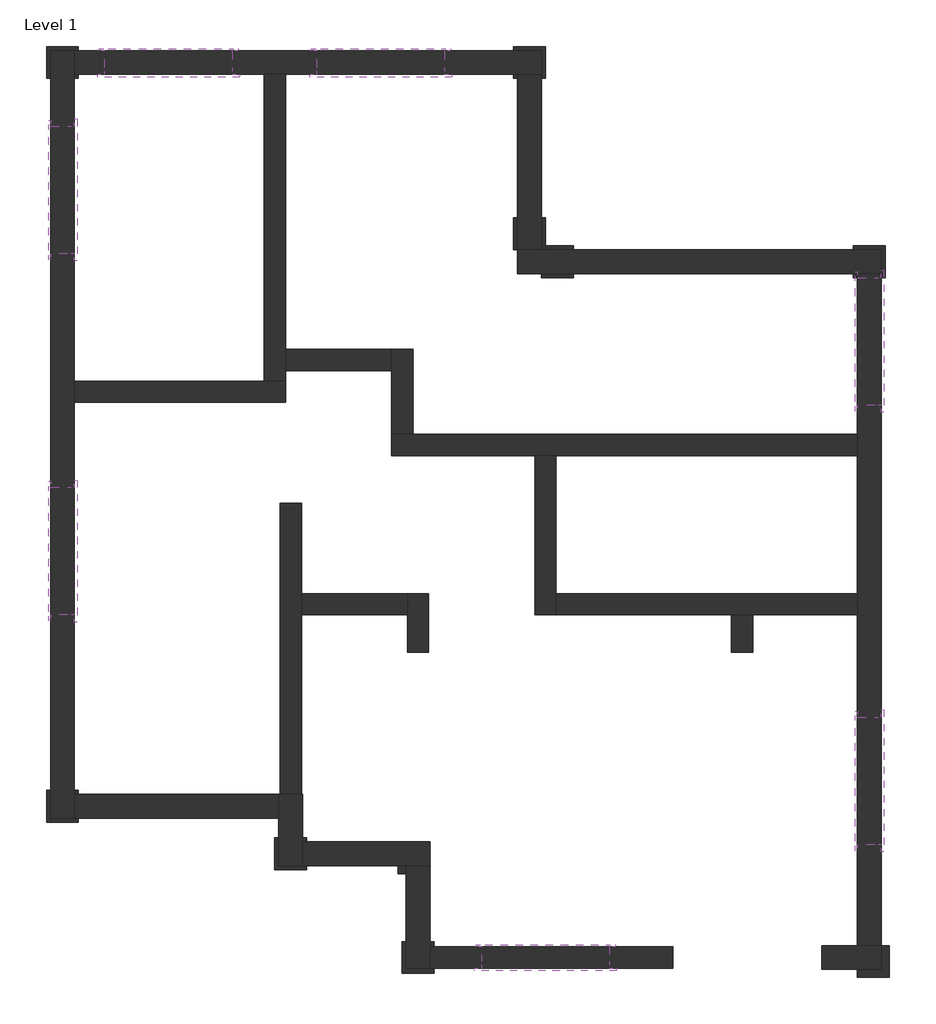
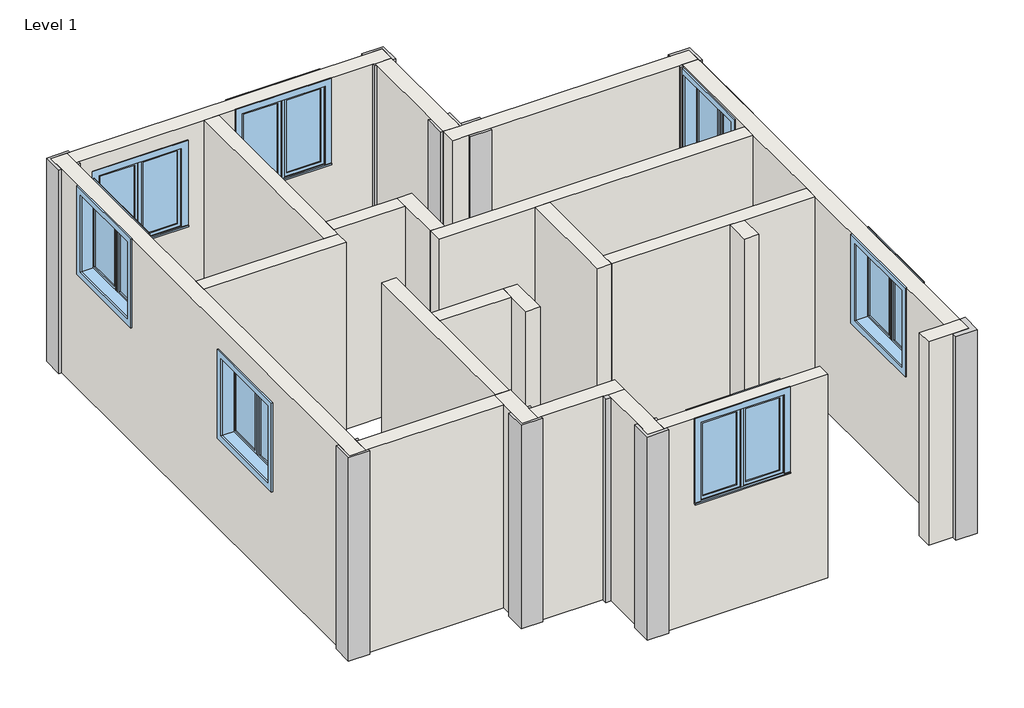
# One storey: 22 walls, 10 columns, 7 windows.
"""IFC4 building model written with IfcOpenShell, lengths in millimetres."""

from ifc_helpers import new_model, si_unit, origin, origin_with_axes, place, context, project, spatial, polyline, outline, extrude, faceted_brep, transform, mapped, element, save
from components import window_534dcd48, window_0862ab64

model = new_model("IFC4")

# Units and contexts
model_context = context("Model", 3, world=origin())
ifc_project = project(units=[si_unit("LENGTHUNIT", "METRE", prefix="MILLI")], contexts=[model_context])

# Site, building, storey
site = spatial("IfcSite", under=ifc_project)
building = spatial("IfcBuilding", under=site)
storey = spatial("IfcBuildingStorey", under=building, Name="Level 1", Elevation=0.0)

# Columns
placement = place(None, origin())
element("IfcColumn", 1, ObjectType="Rectangular Column : 12\" x 12\"", at=placement, inside=storey, context=model_context, shape_type="SweptSolid", body=[
    extrude(outline(polyline([(-12153.373418, 12563.7966667), (-12115.273418, 12563.7966667), (-12115.273418, 12525.6966667), (-12153.373418, 12525.6966667), (-12153.373418, 12563.7966667)])), origin_with_axes(), (0.0, 0.0, 1.0), 3048.0),
    extrude(outline(polyline([(-12115.273418, 12258.9966667), (-12420.073418, 12258.9966667), (-12420.073418, 12563.7966667), (-12381.973418, 12563.7966667), (-12381.973418, 12297.0966667), (-12153.373418, 12297.0966667), (-12115.273418, 12297.0966667), (-12115.273418, 12258.9966667)])), origin_with_axes(), (0.0, 0.0, 1.0), 3048.0),
])
element("IfcColumn", 2, ObjectType="Rectangular Column : 12\" x 12\"", at=placement, inside=storey, context=model_context, shape_type="SweptSolid", body=[
    extrude(outline(polyline([(-9968.973418, 12106.5966667), (-9930.873418, 12106.5966667), (-9930.873418, 12068.4966667), (-9968.973418, 12068.4966667), (-9968.973418, 12106.5966667)])), origin_with_axes(), (0.0, 0.0, 1.0), 3048.0),
    extrude(outline(polyline([(-9930.873418, 11801.7966667), (-10235.673418, 11801.7966667), (-10235.673418, 12106.5966667), (-10197.573418, 12106.5966667), (-10197.573418, 11839.8966667), (-9968.973418, 11839.8966667), (-9930.873418, 11839.8966667), (-9930.873418, 11801.7966667)])), origin_with_axes(), (0.0, 0.0, 1.0), 3048.0),
])
element("IfcColumn", 3, ObjectType="Rectangular Column : 12\" x 12\"", at=placement, inside=storey, context=model_context, shape_type="SweptSolid", body=[
    extrude(outline(polyline([(-4355.573418, 11077.8966667), (-4355.573418, 10773.0966667), (-4660.373418, 10773.0966667), (-4660.373418, 10849.2966667), (-4431.773418, 10849.2966667), (-4431.773418, 11077.8966667), (-4355.573418, 11077.8966667)])), origin_with_axes(), (0.0, 0.0, 1.0), 3048.0),
])
element("IfcColumn", 4, ObjectType="Rectangular Column : 12\" x 12\"", at=placement, inside=storey, context=model_context, shape_type="SweptSolid", body=[
    extrude(outline(polyline([(-9054.573418, 11763.6966667), (-9054.573418, 11839.8966667), (-8978.373418, 11839.8966667), (-8978.373418, 11763.6966667), (-9054.573418, 11763.6966667)])), origin_with_axes(), (0.0, 0.0, 1.0), 3048.0),
])
element("IfcColumn", 5, ObjectType="Rectangular Column : 12\" x 12\"", at=placement, inside=storey, context=model_context, shape_type="SweptSolid", body=[
    extrude(outline(polyline([(-12420.073418, 19370.9966667), (-12420.073418, 19675.7966667), (-12115.273418, 19675.7966667), (-12115.273418, 19637.6966667), (-12153.373418, 19637.6966667), (-12381.973418, 19637.6966667), (-12381.973418, 19370.9966667), (-12420.073418, 19370.9966667)])), origin_with_axes(), (0.0, 0.0, 1.0), 3048.0),
    extrude(outline(polyline([(-12115.273418, 19370.9966667), (-12153.373418, 19370.9966667), (-12153.373418, 19409.0966667), (-12115.273418, 19409.0966667), (-12115.273418, 19370.9966667)])), origin_with_axes(), (0.0, 0.0, 1.0), 3048.0),
])
element("IfcColumn", 6, ObjectType="Rectangular Column : 12\" x 12\"", at=placement, inside=storey, context=model_context, shape_type="SweptSolid", body=[
    extrude(outline(polyline([(-7949.673418, 19370.9966667), (-7949.673418, 19409.0966667), (-7911.573418, 19409.0966667), (-7911.573418, 19370.9966667), (-7949.673418, 19370.9966667)])), origin_with_axes(), (0.0, 0.0, 1.0), 3048.0),
    extrude(outline(polyline([(-7644.873418, 19675.7966667), (-7644.873418, 19370.9966667), (-7682.973418, 19370.9966667), (-7682.973418, 19409.0966667), (-7682.973418, 19637.6966667), (-7949.673418, 19637.6966667), (-7949.673418, 19675.7966667), (-7644.873418, 19675.7966667)])), origin_with_axes(), (0.0, 0.0, 1.0), 3048.0),
])
element("IfcColumn", 7, ObjectType="Rectangular Column : 12\" x 12\"", at=placement, inside=storey, context=model_context, shape_type="SweptSolid", body=[
    extrude(outline(polyline([(-7949.673418, 17732.6966667), (-7949.673418, 18037.4966667), (-7911.573418, 18037.4966667), (-7911.573418, 17732.6966667), (-7949.673418, 17732.6966667)])), origin_with_axes(), (0.0, 0.0, 1.0), 3048.0),
    extrude(outline(polyline([(-7644.873418, 18037.4966667), (-7644.873418, 17732.6966667), (-7682.973418, 17732.6966667), (-7682.973418, 18037.4966667), (-7644.873418, 18037.4966667)])), origin_with_axes(), (0.0, 0.0, 1.0), 3048.0),
])
element("IfcColumn", 8, ObjectType="Rectangular Column : 12\" x 12\"", at=placement, inside=storey, context=model_context, shape_type="SweptSolid", body=[
    extrude(outline(polyline([(-7682.973418, 17770.7966667), (-7378.173418, 17770.7966667), (-7378.173418, 17732.6966667), (-7682.973418, 17732.6966667), (-7682.973418, 17770.7966667)])), origin_with_axes(), (0.0, 0.0, 1.0), 3048.0),
    extrude(outline(polyline([(-7378.173418, 17465.9966667), (-7682.973418, 17465.9966667), (-7682.973418, 17504.0966667), (-7378.173418, 17504.0966667), (-7378.173418, 17465.9966667)])), origin_with_axes(), (0.0, 0.0, 1.0), 3048.0),
])
element("IfcColumn", 9, ObjectType="Rectangular Column : 12\" x 12\"", at=placement, inside=storey, context=model_context, shape_type="Brep", body=[
    faceted_brep([(-4698.473418, 17465.9966667, 0.0), (-4698.473418, 17504.0966667, 0.0), (-4660.373418, 17504.0966667, 0.0), (-4660.373418, 17465.9966667, 0.0), (-4698.473418, 17465.9966667, 3048.0), (-4660.373418, 17465.9966667, 1752.0661962), (-4660.373418, 17465.9966667, 2971.2661962), (-4660.373418, 17465.9966667, 3048.0), (-4698.473418, 17504.0966667, 3048.0), (-4660.373418, 17504.0966667, 3048.0)], [[[0, 1, 2, 3]], [[4, 0, 3, 5, 6, 7]], [[1, 8, 9, 2]], [[0, 4, 8, 1]], [[3, 2, 9, 7, 6, 5]], [[8, 4, 7, 9]]]),
    faceted_brep([(-4393.673418, 17465.9966667, 0.0), (-4393.673418, 17770.7966667, 0.0), (-4393.673418, 17770.7966667, 3048.0), (-4393.673418, 17465.9966667, 3048.0), (-4698.473418, 17770.7966667, 3048.0), (-4698.473418, 17770.7966667, 0.0), (-4698.473418, 17732.6966667, 0.0), (-4698.473418, 17732.6966667, 3048.0), (-4431.773418, 17732.6966667, 3048.0), (-4431.773418, 17504.0966667, 3048.0), (-4431.773418, 17465.9966667, 3048.0), (-4431.773418, 17732.6966667, 0.0), (-4431.773418, 17504.0966667, 0.0), (-4431.773418, 17465.9966667, 0.0), (-4431.773418, 17465.9966667, 1752.0661962), (-4431.773418, 17465.9966667, 2971.2661962)], [[[0, 1, 2, 3]], [[4, 5, 6, 7]], [[1, 5, 4, 2]], [[3, 2, 4, 7, 8, 9, 10]], [[11, 8, 7, 6]], [[8, 11, 12, 9]], [[12, 13, 14, 15, 10, 9]], [[1, 0, 13, 12, 11, 6, 5]], [[0, 3, 10, 15, 14, 13]]]),
])
element("IfcColumn", 10, ObjectType="Rectangular Column : 12\" x 12\"", at=placement, inside=storey, context=model_context, shape_type="SweptSolid", body=[
    extrude(outline(polyline([(-8749.773418, 11115.9966667), (-8711.673418, 11115.9966667), (-8711.673418, 11065.1966667), (-8749.773418, 11065.1966667), (-8749.773418, 11115.9966667)])), origin_with_axes(), (0.0, 0.0, 1.0), 3048.0),
    extrude(outline(polyline([(-8711.673418, 10811.1966667), (-9016.473418, 10811.1966667), (-9016.473418, 11115.9966667), (-8978.373418, 11115.9966667), (-8978.373418, 10861.9966667), (-8749.773418, 10861.9966667), (-8711.673418, 10861.9966667), (-8711.673418, 10811.1966667)])), origin_with_axes(), (0.0, 0.0, 1.0), 3048.0),
])

# Walls
element("IfcWall", 11, ObjectType="Generic - 8\"", at=placement, inside=storey, context=model_context, shape_type="Brep", body=[
    faceted_brep([(-10134.073418, 16475.3966667, 0.0), (-10134.073418, 16576.9966667, 0.0), (-10134.073418, 16780.1966667, 0.0), (-10134.073418, 19409.0966667, 0.0), (-10134.073418, 19409.0966667, 3048.0), (-10134.073418, 16780.1966667, 3048.0), (-10134.073418, 16576.9966667, 3048.0), (-10134.073418, 16475.3966667, 3048.0), (-10337.273418, 16475.3966667, 0.0), (-10337.273418, 16475.3966667, 3048.0), (-10337.273418, 19409.0966667, 3048.0), (-10337.273418, 19409.0966667, 0.0)], [[[0, 1, 2, 3, 4, 5, 6, 7]], [[8, 9, 10, 11]], [[3, 2, 1, 0, 8, 11]], [[7, 6, 5, 4, 10, 9]], [[0, 7, 9, 8]], [[4, 3, 11, 10]]]),
])
element("IfcWall", 12, ObjectType="Generic - 8\"", at=placement, inside=storey, context=model_context, shape_type="Brep", body=[
    faceted_brep([(-12153.373418, 16272.1966667, 0.0), (-10134.073418, 16272.1966667, 0.0), (-10134.073418, 16272.1966667, 3048.0), (-12153.373418, 16272.1966667, 3048.0), (-12153.373418, 16475.3966667, 0.0), (-12153.373418, 16475.3966667, 3048.0), (-10337.273418, 16475.3966667, 3048.0), (-10134.073418, 16475.3966667, 3048.0), (-10134.073418, 16475.3966667, 0.0), (-10337.273418, 16475.3966667, 0.0)], [[[0, 1, 2, 3]], [[4, 5, 6, 7, 8, 9]], [[1, 0, 4, 9, 8]], [[3, 2, 7, 6, 5]], [[2, 1, 8, 7]], [[0, 3, 5, 4]]]),
])
element("IfcWall", 13, ObjectType="Generic - 8\"", at=placement, inside=storey, context=model_context, shape_type="Brep", body=[
    faceted_brep([(-4660.373418, 15967.3966667, 0.0), (-8914.873418, 15967.3966667, 0.0), (-9118.073418, 15967.3966667, 0.0), (-9118.073418, 15967.3966667, 3048.0), (-8914.873418, 15967.3966667, 3048.0), (-4660.373418, 15967.3966667, 3048.0), (-4660.373418, 15764.1966667, 0.0), (-4660.373418, 15764.1966667, 3048.0), (-7543.273418, 15764.1966667, 3048.0), (-7746.473418, 15764.1966667, 3048.0), (-9118.073418, 15764.1966667, 3048.0), (-9118.073418, 15764.1966667, 0.0), (-7746.473418, 15764.1966667, 0.0), (-7543.273418, 15764.1966667, 0.0)], [[[0, 1, 2, 3, 4, 5]], [[6, 7, 8, 9, 10, 11, 12, 13]], [[2, 1, 0, 6, 13, 12, 11]], [[5, 4, 3, 10, 9, 8, 7]], [[3, 2, 11, 10]], [[0, 5, 7, 6]]]),
])
element("IfcWall", 14, ObjectType="Generic - 8\"", at=placement, inside=storey, context=model_context, shape_type="Brep", body=[
    faceted_brep([(-8914.873418, 15967.3966667, 0.0), (-8914.873418, 16780.1966667, 0.0), (-8914.873418, 16780.1966667, 3048.0), (-8914.873418, 15967.3966667, 3048.0), (-9118.073418, 15967.3966667, 0.0), (-9118.073418, 15967.3966667, 3048.0), (-9118.073418, 16576.9966667, 3048.0), (-9118.073418, 16780.1966667, 3048.0), (-9118.073418, 16780.1966667, 0.0), (-9118.073418, 16576.9966667, 0.0)], [[[0, 1, 2, 3]], [[4, 5, 6, 7, 8, 9]], [[1, 0, 4, 9, 8]], [[3, 2, 7, 6, 5]], [[0, 3, 5, 4]], [[2, 1, 8, 7]]]),
])
element("IfcWall", 15, ObjectType="Generic - 8\"", at=placement, inside=storey, context=model_context, shape_type="SweptSolid", body=[
    extrude(outline(polyline([(-10134.073418, 16780.1966667), (-9118.073418, 16780.1966667), (-9118.073418, 16576.9966667), (-10134.073418, 16576.9966667), (-10134.073418, 16780.1966667)])), origin_with_axes(), (0.0, 0.0, 1.0), 3048.0),
])
element("IfcWall", 16, ObjectType="Generic - 8\"", at=placement, inside=storey, context=model_context, shape_type="SweptSolid", body=[
    extrude(outline(polyline([(-8965.673418, 14240.1966667), (-9981.673418, 14240.1966667), (-9981.673418, 14443.3966667), (-8965.673418, 14443.3966667), (-8965.673418, 14240.1966667)])), origin_with_axes(), (0.0, 0.0, 1.0), 3048.0),
])
element("IfcWall", 17, ObjectType="Generic - 8\"", at=placement, inside=storey, context=model_context, shape_type="Brep", body=[
    faceted_brep([(-8965.673418, 14443.3966667, 0.0), (-8965.673418, 14240.1966667, 0.0), (-8965.673418, 13884.5966667, 0.0), (-8965.673418, 13884.5966667, 3048.0), (-8965.673418, 14240.1966667, 3048.0), (-8965.673418, 14443.3966667, 3048.0), (-8762.473418, 14443.3966667, 0.0), (-8762.473418, 14443.3966667, 3048.0), (-8762.473418, 13884.5966667, 3048.0), (-8762.473418, 13884.5966667, 0.0)], [[[0, 1, 2, 3, 4, 5]], [[6, 7, 8, 9]], [[2, 1, 0, 6, 9]], [[3, 2, 9, 8]], [[5, 4, 3, 8, 7]], [[0, 5, 7, 6]]]),
])
element("IfcWall", 18, ObjectType="Generic - 8\"", at=placement, inside=storey, context=model_context, shape_type="Brep", body=[
    faceted_brep([(-7746.473418, 15764.1966667, 0.0), (-7746.473418, 14240.1966667, 0.0), (-7746.473418, 14240.1966667, 3048.0), (-7746.473418, 15764.1966667, 3048.0), (-7543.273418, 15764.1966667, 0.0), (-7543.273418, 15764.1966667, 3048.0), (-7543.273418, 14443.3966667, 3048.0), (-7543.273418, 14240.1966667, 3048.0), (-7543.273418, 14240.1966667, 0.0), (-7543.273418, 14443.3966667, 0.0)], [[[0, 1, 2, 3]], [[4, 5, 6, 7, 8, 9]], [[1, 0, 4, 9, 8]], [[3, 2, 7, 6, 5]], [[0, 3, 5, 4]], [[2, 1, 8, 7]]]),
])
element("IfcWall", 19, ObjectType="Generic - 8\"", at=placement, inside=storey, context=model_context, shape_type="Brep", body=[
    faceted_brep([(-7543.273418, 14240.1966667, 0.0), (-5866.873418, 14240.1966667, 0.0), (-5663.673418, 14240.1966667, 0.0), (-4660.373418, 14240.1966667, 0.0), (-4660.373418, 14240.1966667, 3048.0), (-5663.673418, 14240.1966667, 3048.0), (-5866.873418, 14240.1966667, 3048.0), (-7543.273418, 14240.1966667, 3048.0), (-7543.273418, 14443.3966667, 0.0), (-7543.273418, 14443.3966667, 3048.0), (-4660.373418, 14443.3966667, 3048.0), (-4660.373418, 14443.3966667, 0.0)], [[[0, 1, 2, 3, 4, 5, 6, 7]], [[8, 9, 10, 11]], [[3, 2, 1, 0, 8, 11]], [[7, 6, 5, 4, 10, 9]], [[0, 7, 9, 8]], [[4, 3, 11, 10]]]),
])
element("IfcWall", 20, ObjectType="Generic - 8\"", at=placement, inside=storey, context=model_context, shape_type="SweptSolid", body=[
    extrude(outline(polyline([(-5866.873418, 13884.5966667), (-5866.873418, 14240.1966667), (-5663.673418, 14240.1966667), (-5663.673418, 13884.5966667), (-5866.873418, 13884.5966667)])), origin_with_axes(), (0.0, 0.0, 1.0), 3048.0),
])
element("IfcWall", 21, ObjectType="Generic - 8\"", at=placement, inside=storey, context=model_context, shape_type="Brep", body=[
    faceted_brep([(-9981.673418, 12525.6966667, 0.0), (-9981.673418, 14240.1966667, 0.0), (-9981.673418, 14443.3966667, 0.0), (-9981.673418, 15306.9966667, 0.0), (-9981.673418, 15306.9966667, 3048.0), (-9981.673418, 14443.3966667, 3048.0), (-9981.673418, 14240.1966667, 3048.0), (-9981.673418, 12525.6966667, 3048.0), (-10184.873418, 12525.6966667, 0.0), (-10184.873418, 12525.6966667, 3048.0), (-10184.873418, 15306.9966667, 3048.0), (-10184.873418, 15306.9966667, 0.0)], [[[0, 1, 2, 3, 4, 5, 6, 7]], [[8, 9, 10, 11]], [[3, 2, 1, 0, 8, 11]], [[4, 3, 11, 10]], [[7, 6, 5, 4, 10, 9]], [[0, 7, 9, 8]]]),
])
element("IfcWall", 22, ObjectType="Generic - 8\"", at=placement, inside=storey, context=model_context, shape_type="Brep", body=[
    faceted_brep([(-8749.773418, 10861.9966667, 0.0), (-8711.673418, 10861.9966667, 0.0), (-6425.673418, 10861.9966667, 0.0), (-6425.673418, 10861.9966667, 3048.0), (-8711.673418, 10861.9966667, 3048.0), (-8749.773418, 10861.9966667, 3048.0), (-8254.473418, 10861.9966667, 1770.781986), (-8254.473418, 10861.9966667, 2989.981986), (-7035.273418, 10861.9966667, 2989.981986), (-7035.273418, 10861.9966667, 1770.781986), (-6425.673418, 11065.1966667, 0.0), (-8711.673418, 11065.1966667, 0.0), (-8749.773418, 11065.1966667, 0.0), (-8749.773418, 11065.1966667, 3048.0), (-8711.673418, 11065.1966667, 3048.0), (-6425.673418, 11065.1966667, 3048.0), (-8254.473418, 11065.1966667, 2989.981986), (-8254.473418, 11065.1966667, 1770.781986), (-7035.273418, 11065.1966667, 1770.781986), (-7035.273418, 11065.1966667, 2989.981986)], [[[0, 1, 2, 3, 4, 5], [6, 7, 8, 9]], [[10, 11, 12, 13, 14, 15], [16, 17, 18, 19]], [[2, 1, 0, 12, 11, 10]], [[3, 2, 10, 15]], [[5, 4, 3, 15, 14, 13]], [[0, 5, 13, 12]], [[16, 7, 6, 17]], [[17, 6, 9, 18]], [[18, 9, 8, 19]], [[7, 16, 19, 8]]]),
])
element("IfcWall", 23, ObjectType="Generic - 9\"", at=placement, inside=storey, context=model_context, shape_type="Brep", body=[
    faceted_brep([(-12153.373418, 12297.0966667, 0.0), (-12153.373418, 12525.6966667, 0.0), (-12153.373418, 12563.7966667, 0.0), (-12153.373418, 16272.1966667, 0.0), (-12153.373418, 16475.3966667, 0.0), (-12153.373418, 19370.9966667, 0.0), (-12153.373418, 19409.0966667, 0.0), (-12153.373418, 19637.6966667, 0.0), (-12153.373418, 19637.6966667, 3048.0), (-12153.373418, 19409.0966667, 3048.0), (-12153.373418, 19370.9966667, 3048.0), (-12153.373418, 16475.3966667, 3048.0), (-12153.373418, 16272.1966667, 3048.0), (-12153.373418, 12563.7966667, 3048.0), (-12153.373418, 12525.6966667, 3048.0), (-12153.373418, 12297.0966667, 3048.0), (-12153.373418, 14240.1966667, 2638.3969911), (-12153.373418, 15459.3966667, 2638.3969911), (-12153.373418, 15459.3966667, 1419.1969911), (-12153.373418, 14240.1966667, 1419.1969911), (-12153.373418, 17694.5966667, 2999.5449591), (-12153.373418, 18913.7966667, 2999.5449591), (-12153.373418, 18913.7966667, 1780.3449591), (-12153.373418, 17694.5966667, 1780.3449591), (-12381.973418, 12297.0966667, 0.0), (-12381.973418, 12297.0966667, 3048.0), (-12381.973418, 12563.7966667, 3048.0), (-12381.973418, 19370.9966667, 3048.0), (-12381.973418, 19637.6966667, 3048.0), (-12381.973418, 19637.6966667, 0.0), (-12381.973418, 19370.9966667, 0.0), (-12381.973418, 12563.7966667, 0.0), (-12381.973418, 14240.1966667, 2638.3969911), (-12381.973418, 14240.1966667, 1419.1969911), (-12381.973418, 15459.3966667, 1419.1969911), (-12381.973418, 15459.3966667, 2638.3969911), (-12381.973418, 17694.5966667, 2999.5449591), (-12381.973418, 17694.5966667, 1780.3449591), (-12381.973418, 18913.7966667, 1780.3449591), (-12381.973418, 18913.7966667, 2999.5449591)], [[[0, 1, 2, 3, 4, 5, 6, 7, 8, 9, 10, 11, 12, 13, 14, 15], [16, 17, 18, 19], [20, 21, 22, 23]], [[24, 25, 26, 27, 28, 29, 30, 31], [32, 33, 34, 35], [36, 37, 38, 39]], [[7, 6, 5, 4, 3, 2, 1, 0, 24, 31, 30, 29]], [[15, 14, 13, 12, 11, 10, 9, 8, 28, 27, 26, 25]], [[8, 7, 29, 28]], [[0, 15, 25, 24]], [[33, 32, 16, 19]], [[34, 33, 19, 18]], [[35, 34, 18, 17]], [[32, 35, 17, 16]], [[37, 36, 20, 23]], [[38, 37, 23, 22]], [[39, 38, 22, 21]], [[36, 39, 21, 20]]]),
])
element("IfcWall", 24, ObjectType="Generic - 9\"", at=placement, inside=storey, context=model_context, shape_type="Brep", body=[
    faceted_brep([(-12153.373418, 19409.0966667, 0.0), (-12115.273418, 19409.0966667, 0.0), (-10337.273418, 19409.0966667, 0.0), (-10134.073418, 19409.0966667, 0.0), (-7949.673418, 19409.0966667, 0.0), (-7911.573418, 19409.0966667, 0.0), (-7682.973418, 19409.0966667, 0.0), (-7682.973418, 19409.0966667, 3048.0), (-7911.573418, 19409.0966667, 3048.0), (-7949.673418, 19409.0966667, 3048.0), (-10134.073418, 19409.0966667, 3048.0), (-10337.273418, 19409.0966667, 3048.0), (-12115.273418, 19409.0966667, 3048.0), (-12153.373418, 19409.0966667, 3048.0), (-11861.273418, 19409.0966667, 2768.0733657), (-10642.073418, 19409.0966667, 2768.0733657), (-10642.073418, 19409.0966667, 1548.8733657), (-11861.273418, 19409.0966667, 1548.8733657), (-9829.273418, 19409.0966667, 2987.4864243), (-8610.073418, 19409.0966667, 2987.4864243), (-8610.073418, 19409.0966667, 1768.2864243), (-9829.273418, 19409.0966667, 1768.2864243), (-12153.373418, 19637.6966667, 0.0), (-12153.373418, 19637.6966667, 3048.0), (-12115.273418, 19637.6966667, 3048.0), (-7949.673418, 19637.6966667, 3048.0), (-7682.973418, 19637.6966667, 3048.0), (-7682.973418, 19637.6966667, 0.0), (-7949.673418, 19637.6966667, 0.0), (-12115.273418, 19637.6966667, 0.0), (-11861.273418, 19637.6966667, 2768.0733657), (-11861.273418, 19637.6966667, 1548.8733657), (-10642.073418, 19637.6966667, 1548.8733657), (-10642.073418, 19637.6966667, 2768.0733657), (-9829.273418, 19637.6966667, 2987.4864243), (-9829.273418, 19637.6966667, 1768.2864243), (-8610.073418, 19637.6966667, 1768.2864243), (-8610.073418, 19637.6966667, 2987.4864243)], [[[0, 1, 2, 3, 4, 5, 6, 7, 8, 9, 10, 11, 12, 13], [14, 15, 16, 17], [18, 19, 20, 21]], [[22, 23, 24, 25, 26, 27, 28, 29], [30, 31, 32, 33], [34, 35, 36, 37]], [[6, 5, 4, 3, 2, 1, 0, 22, 29, 28, 27]], [[13, 12, 11, 10, 9, 8, 7, 26, 25, 24, 23]], [[0, 13, 23, 22]], [[7, 6, 27, 26]], [[31, 30, 14, 17]], [[32, 31, 17, 16]], [[33, 32, 16, 15]], [[30, 33, 15, 14]], [[35, 34, 18, 21]], [[36, 35, 21, 20]], [[37, 36, 20, 19]], [[34, 37, 19, 18]]]),
])
element("IfcWall", 25, ObjectType="Generic - 9\"", at=placement, inside=storey, context=model_context, shape_type="Brep", body=[
    faceted_brep([(-7911.573418, 19409.0966667, 0.0), (-7911.573418, 19370.9966667, 0.0), (-7911.573418, 18037.4966667, 0.0), (-7911.573418, 17732.6966667, 0.0), (-7911.573418, 17732.6966667, 3048.0), (-7911.573418, 18037.4966667, 3048.0), (-7911.573418, 19370.9966667, 3048.0), (-7911.573418, 19409.0966667, 3048.0), (-7682.973418, 19409.0966667, 0.0), (-7682.973418, 19409.0966667, 3048.0), (-7682.973418, 19370.9966667, 3048.0), (-7682.973418, 18037.4966667, 3048.0), (-7682.973418, 17770.7966667, 3048.0), (-7682.973418, 17732.6966667, 3048.0), (-7682.973418, 17732.6966667, 0.0), (-7682.973418, 17770.7966667, 0.0), (-7682.973418, 18037.4966667, 0.0), (-7682.973418, 19370.9966667, 0.0)], [[[0, 1, 2, 3, 4, 5, 6, 7]], [[8, 9, 10, 11, 12, 13, 14, 15, 16, 17]], [[3, 2, 1, 0, 8, 17, 16, 15, 14]], [[7, 6, 5, 4, 13, 12, 11, 10, 9]], [[0, 7, 9, 8]], [[4, 3, 14, 13]]]),
])
element("IfcWall", 26, ObjectType="Generic - 9\"", at=placement, inside=storey, context=model_context, shape_type="Brep", body=[
    faceted_brep([(-4431.773418, 17732.6966667, 0.0), (-4698.473418, 17732.6966667, 0.0), (-7378.173418, 17732.6966667, 0.0), (-7644.873418, 17732.6966667, 0.0), (-7682.973418, 17732.6966667, 0.0), (-7911.573418, 17732.6966667, 0.0), (-7911.573418, 17732.6966667, 3048.0), (-7682.973418, 17732.6966667, 3048.0), (-7644.873418, 17732.6966667, 3048.0), (-7378.173418, 17732.6966667, 3048.0), (-4698.473418, 17732.6966667, 3048.0), (-4431.773418, 17732.6966667, 3048.0), (-4431.773418, 17504.0966667, 0.0), (-4431.773418, 17504.0966667, 3048.0), (-4660.373418, 17504.0966667, 3048.0), (-4698.473418, 17504.0966667, 3048.0), (-7378.173418, 17504.0966667, 3048.0), (-7682.973418, 17504.0966667, 3048.0), (-7911.573418, 17504.0966667, 3048.0), (-7911.573418, 17504.0966667, 0.0), (-7682.973418, 17504.0966667, 0.0), (-7378.173418, 17504.0966667, 0.0), (-4698.473418, 17504.0966667, 0.0), (-4660.373418, 17504.0966667, 0.0)], [[[0, 1, 2, 3, 4, 5, 6, 7, 8, 9, 10, 11]], [[12, 13, 14, 15, 16, 17, 18, 19, 20, 21, 22, 23]], [[5, 4, 3, 2, 1, 0, 12, 23, 22, 21, 20, 19]], [[11, 10, 9, 8, 7, 6, 18, 17, 16, 15, 14, 13]], [[6, 5, 19, 18]], [[0, 11, 13, 12]]]),
])
element("IfcWall", 27, ObjectType="Generic - 9\"", at=placement, inside=storey, context=model_context, shape_type="Brep", body=[
    faceted_brep([(-12153.373418, 12297.0966667, 0.0), (-12115.273418, 12297.0966667, 0.0), (-10197.573418, 12297.0966667, 0.0), (-10197.573418, 12297.0966667, 3048.0), (-12115.273418, 12297.0966667, 3048.0), (-12153.373418, 12297.0966667, 3048.0), (-12153.373418, 12525.6966667, 0.0), (-12153.373418, 12525.6966667, 3048.0), (-12115.273418, 12525.6966667, 3048.0), (-10197.573418, 12525.6966667, 3048.0), (-10197.573418, 12525.6966667, 0.0), (-12115.273418, 12525.6966667, 0.0)], [[[0, 1, 2, 3, 4, 5]], [[6, 7, 8, 9, 10, 11]], [[2, 1, 0, 6, 11, 10]], [[5, 4, 3, 9, 8, 7]], [[0, 5, 7, 6]], [[3, 2, 10, 9]]]),
])
element("IfcWall", 28, ObjectType="Generic - 9\"", at=placement, inside=storey, context=model_context, shape_type="Brep", body=[
    faceted_brep([(-9968.973418, 11839.8966667, 0.0), (-9968.973418, 12068.4966667, 0.0), (-9968.973418, 12106.5966667, 0.0), (-9968.973418, 12525.6966667, 0.0), (-9968.973418, 12525.6966667, 3048.0), (-9968.973418, 12106.5966667, 3048.0), (-9968.973418, 12068.4966667, 3048.0), (-9968.973418, 11839.8966667, 3048.0), (-10197.573418, 11839.8966667, 0.0), (-10197.573418, 11839.8966667, 3048.0), (-10197.573418, 12106.5966667, 3048.0), (-10197.573418, 12297.0966667, 3048.0), (-10197.573418, 12525.6966667, 3048.0), (-10197.573418, 12525.6966667, 0.0), (-10197.573418, 12297.0966667, 0.0), (-10197.573418, 12106.5966667, 0.0), (-10184.873418, 12525.6966667, 0.0), (-9981.673418, 12525.6966667, 0.0), (-9981.673418, 12525.6966667, 3048.0), (-10184.873418, 12525.6966667, 3048.0)], [[[0, 1, 2, 3, 4, 5, 6, 7]], [[8, 9, 10, 11, 12, 13, 14, 15]], [[3, 2, 1, 0, 8, 15, 14, 13, 16, 17]], [[7, 6, 5, 4, 18, 19, 12, 11, 10, 9]], [[0, 7, 9, 8]], [[4, 3, 17, 16, 13, 12, 19, 18]]]),
])
element("IfcWall", 29, ObjectType="Generic - 9\"", at=placement, inside=storey, context=model_context, shape_type="Brep", body=[
    faceted_brep([(-9968.973418, 11839.8966667, 0.0), (-9930.873418, 11839.8966667, 0.0), (-9054.573418, 11839.8966667, 0.0), (-8978.373418, 11839.8966667, 0.0), (-8749.773418, 11839.8966667, 0.0), (-8749.773418, 11839.8966667, 3048.0), (-8978.373418, 11839.8966667, 3048.0), (-9054.573418, 11839.8966667, 3048.0), (-9930.873418, 11839.8966667, 3048.0), (-9968.973418, 11839.8966667, 3048.0), (-9968.973418, 12068.4966667, 0.0), (-9968.973418, 12068.4966667, 3048.0), (-9930.873418, 12068.4966667, 3048.0), (-8749.773418, 12068.4966667, 3048.0), (-8749.773418, 12068.4966667, 0.0), (-9930.873418, 12068.4966667, 0.0)], [[[0, 1, 2, 3, 4, 5, 6, 7, 8, 9]], [[10, 11, 12, 13, 14, 15]], [[4, 3, 2, 1, 0, 10, 15, 14]], [[9, 8, 7, 6, 5, 13, 12, 11]], [[5, 4, 14, 13]], [[0, 9, 11, 10]]]),
])
element("IfcWall", 30, ObjectType="Generic - 9\"", at=placement, inside=storey, context=model_context, shape_type="Brep", body=[
    faceted_brep([(-8978.373418, 11839.8966667, 0.0), (-8978.373418, 11763.6966667, 0.0), (-8978.373418, 11115.9966667, 0.0), (-8978.373418, 10861.9966667, 0.0), (-8978.373418, 10861.9966667, 3048.0), (-8978.373418, 11115.9966667, 3048.0), (-8978.373418, 11763.6966667, 3048.0), (-8978.373418, 11839.8966667, 3048.0), (-8749.773418, 11839.8966667, 0.0), (-8749.773418, 11839.8966667, 3048.0), (-8749.773418, 11115.9966667, 3048.0), (-8749.773418, 11065.1966667, 3048.0), (-8749.773418, 10861.9966667, 3048.0), (-8749.773418, 10861.9966667, 0.0), (-8749.773418, 11065.1966667, 0.0), (-8749.773418, 11115.9966667, 0.0)], [[[0, 1, 2, 3, 4, 5, 6, 7]], [[8, 9, 10, 11, 12, 13, 14, 15]], [[3, 2, 1, 0, 8, 15, 14, 13]], [[7, 6, 5, 4, 12, 11, 10, 9]], [[0, 7, 9, 8]], [[4, 3, 13, 12]]]),
])
element("IfcWall", 31, ObjectType="Generic - 9\"", at=placement, inside=storey, context=model_context, shape_type="Brep", body=[
    faceted_brep([(-5003.273418, 10849.2966667, 0.0), (-4660.373418, 10849.2966667, 0.0), (-4431.773418, 10849.2966667, 0.0), (-4431.773418, 10849.2966667, 3048.0), (-4660.373418, 10849.2966667, 3048.0), (-5003.273418, 10849.2966667, 3048.0), (-5003.273418, 11077.8966667, 0.0), (-5003.273418, 11077.8966667, 3048.0), (-4660.373418, 11077.8966667, 3048.0), (-4431.773418, 11077.8966667, 3048.0), (-4431.773418, 11077.8966667, 0.0), (-4660.373418, 11077.8966667, 0.0)], [[[0, 1, 2, 3, 4, 5]], [[6, 7, 8, 9, 10, 11]], [[2, 1, 0, 6, 11, 10]], [[5, 4, 3, 9, 8, 7]], [[0, 5, 7, 6]], [[3, 2, 10, 9]]]),
])
element("IfcWall", 32, ObjectType="Generic - 9\"", at=placement, inside=storey, context=model_context, shape_type="Brep", body=[
    faceted_brep([(-4660.373418, 17504.0966667, 0.0), (-4660.373418, 17465.9966667, 0.0), (-4660.373418, 15967.3966667, 0.0), (-4660.373418, 15764.1966667, 0.0), (-4660.373418, 14443.3966667, 0.0), (-4660.373418, 14240.1966667, 0.0), (-4660.373418, 11077.8966667, 0.0), (-4660.373418, 11077.8966667, 3048.0), (-4660.373418, 14240.1966667, 3048.0), (-4660.373418, 14443.3966667, 3048.0), (-4660.373418, 15764.1966667, 3048.0), (-4660.373418, 15967.3966667, 3048.0), (-4660.373418, 17465.9966667, 3048.0), (-4660.373418, 17504.0966667, 3048.0), (-4660.373418, 12043.0966667, 2994.4957804), (-4660.373418, 12043.0966667, 1775.2957804), (-4660.373418, 13262.2966667, 1775.2957804), (-4660.373418, 13262.2966667, 2994.4957804), (-4660.373418, 16246.7966667, 2971.2661962), (-4660.373418, 16246.7966667, 1752.0661962), (-4660.373418, 17465.9966667, 1752.0661962), (-4660.373418, 17465.9966667, 2971.2661962), (-4431.773418, 17504.0966667, 0.0), (-4431.773418, 17504.0966667, 3048.0), (-4431.773418, 17465.9966667, 3048.0), (-4431.773418, 11077.8966667, 3048.0), (-4431.773418, 11077.8966667, 0.0), (-4431.773418, 17465.9966667, 0.0), (-4431.773418, 12043.0966667, 2994.4957804), (-4431.773418, 13262.2966667, 2994.4957804), (-4431.773418, 13262.2966667, 1775.2957804), (-4431.773418, 12043.0966667, 1775.2957804), (-4431.773418, 16246.7966667, 2971.2661962), (-4431.773418, 17465.9966667, 2971.2661962), (-4431.773418, 17465.9966667, 1752.0661962), (-4431.773418, 16246.7966667, 1752.0661962)], [[[0, 1, 2, 3, 4, 5, 6, 7, 8, 9, 10, 11, 12, 13], [14, 15, 16, 17], [18, 19, 20, 21]], [[22, 23, 24, 25, 26, 27], [28, 29, 30, 31], [32, 33, 34, 35]], [[6, 5, 4, 3, 2, 1, 0, 22, 27, 26]], [[13, 12, 11, 10, 9, 8, 7, 25, 24, 23]], [[0, 13, 23, 22]], [[7, 6, 26, 25]], [[15, 14, 28, 31]], [[16, 15, 31, 30]], [[17, 16, 30, 29]], [[14, 17, 29, 28]], [[19, 18, 32, 35]], [[20, 19, 35, 34]], [[21, 20, 34, 33]], [[18, 21, 33, 32]]]),
])

# Windows
window_shape = window_534dcd48(model_context)
element("IfcWindow", 33, ObjectType="Casement Dbl with Trim : 48\" x 48\"", at=placement, inside=storey, context=model_context, shape_type="MappedRepresentation", body=[
    mapped(window_shape, transform((-4565.123418, 12652.6966667, 860.8957804), x_axis=(0.0, -1.0, 0.0), y_axis=(1.0, 0.0, 0.0), z_axis=(0.0, 0.0, 1.0))),
])
element("IfcWindow", 34, ObjectType="Casement Dbl with Trim : 48\" x 48\"", at=placement, inside=storey, context=model_context, shape_type="MappedRepresentation", body=[
    mapped(window_shape, transform((-12286.723418, 14849.7966667, 504.7969911), x_axis=(0.0, -1.0, 0.0), y_axis=(1.0, 0.0, 0.0), z_axis=(0.0, 0.0, 1.0))),
])
element("IfcWindow", 35, ObjectType="Casement Dbl with Trim : 48\" x 48\"", at=placement, inside=storey, context=model_context, shape_type="MappedRepresentation", body=[
    mapped(window_shape, transform((-12286.723418, 18304.1966667, 865.9449591), x_axis=(0.0, -1.0, 0.0), y_axis=(1.0, 0.0, 0.0), z_axis=(0.0, 0.0, 1.0))),
])
element("IfcWindow", 36, ObjectType="Casement Dbl with Trim : 48\" x 48\"", at=placement, inside=storey, context=model_context, shape_type="MappedRepresentation", body=[
    mapped(window_shape, transform((-11251.673418, 19542.4466667, 634.4733657), x_axis=(-1.0, 0.0, 0.0), y_axis=(0.0, -1.0, 0.0), z_axis=(0.0, 0.0, 1.0))),
])
element("IfcWindow", 37, ObjectType="Casement Dbl with Trim : 48\" x 48\"", at=placement, inside=storey, context=model_context, shape_type="MappedRepresentation", body=[
    mapped(window_shape, transform((-9219.673418, 19542.4466667, 853.8864243), x_axis=(-1.0, 0.0, 0.0), y_axis=(0.0, -1.0, 0.0), z_axis=(0.0, 0.0, 1.0))),
])
element("IfcWindow", 38, ObjectType="Casement Dbl with Trim : 48\" x 48\"", at=placement, inside=storey, context=model_context, shape_type="MappedRepresentation", body=[
    mapped(window_shape, transform((-4565.123418, 16856.3966667, 837.6661962), x_axis=(0.0, -1.0, 0.0), y_axis=(1.0, 0.0, 0.0), z_axis=(0.0, 0.0, 1.0))),
])
window_2_shape = window_0862ab64(model_context)
element("IfcWindow", 39, ObjectType="Casement Dbl with Trim : 48\" x 48\"", at=placement, inside=storey, context=model_context, shape_type="MappedRepresentation", body=[
    mapped(window_2_shape, transform((-7644.873418, 10982.6466667, 856.381986), x_axis=(-1.0, 0.0, 0.0), y_axis=(0.0, -1.0, 0.0), z_axis=(0.0, 0.0, 1.0))),
])

save(model, "model.ifc")

# Revit data of these elements
# Type "Rectangular Column : 12\" x 12\""
#   Assembly Code = "B1010200"
#   Depth = 1' - 0"
#   Offset Base = 0' - 0"
#   Offset Top = 0' - 0"
#   Width = 1' - 0"
#   built-in parameter 1002110 = 6908265
#   Material = none
# Type "Generic - 8\""
#   Assembly Code = "B2010"
#   Layers, outside or top first: 0' - 8" "Tile, Porcelain, 4in" (function 1)
# Type "Generic - 9\""
#   Assembly Code = "B2010"
#   Layers, outside or top first: 0' - 9" "Tile, Porcelain, 4in" (function 1)
# Type "Casement Dbl with Trim : 48\" x 48\""
#   Type Mark = "10"
#   Construction Type Id = "GSP4R"
#   Assembly Code = "B2020100"
#   Analytic Construction = "1/8 in Pilkington single glazing"
#   Visual Light Transmittance = 0.9
#   Solar Heat Gain Coefficient = 0.78
#   Heat Transfer Coefficient (U) = 0.6496 BTU/(h·ft²·°F)
#   Height = 4' - 0"
#   Default Sill Height = 3' - 0"
#   Trim Projection - Ext. = 0' - 0 1/2"
#   Trim Projection - Int. = 0' - 0 3/4"
#   Trim Width - Exterior = 0' - 3 1/2"
#   Trim Width - Interior = 0' - 3 1/2"
#   Width = 4' - 0"
#   Window Inset = 0' - 0 3/4"
#   Define Thermal Properties by = 1
#   Glass Pane Material = Glass
#   Sash Material = Sash
#   Trim Exterior Material = Trim
#   Trim Interior Material = Trim
#   Wall Closure = (empty or 0)
# Elements 1, 2, 3, 4, 5, 6, 7, 8, 9, 10 (IfcColumn, "Rectangular Column : 12\" x 12\"")
#   Phase Created = New Construction
#   Materials on its faces: "Tile, Porcelain, 4in"
# Elements 11, 12, 13, 14, 15, 16, 17, 18, 19, 20, 21, 22 (IfcWall, "Generic - 8\"")
#   Top Offset = 0' - 0"
#   Base Offset = 0' - 0"
#   Unconnected Height = 10' - 0"
#   wall height = 10' - 0"
#   Phase Created = New Construction
#   Base Constraint = Level 1
#   Materials on its faces: "Tile, Porcelain, 4in"
# Elements 23, 24, 25, 26, 27, 28, 29, 30, 31, 32 (IfcWall, "Generic - 9\"")
#   Top Offset = 0' - 0"
#   Base Offset = 0' - 0"
#   Unconnected Height = 10' - 0"
#   wall height = 10' - 0"
#   Phase Created = New Construction
#   Base Constraint = Level 1
#   Materials on its faces: "Tile, Porcelain, 4in"
# Element 33 (IfcWindow, "Casement Dbl with Trim : 48\" x 48\"")
#   Mark = "1"
#   Phase Created = New Construction
#   Materials on its faces: "Sash", "Trim", "Glass"
# Element 34 (IfcWindow, "Casement Dbl with Trim : 48\" x 48\"")
#   Mark = "3"
#   Phase Created = New Construction
#   Materials on its faces: "Sash", "Trim", "Glass"
# Element 35 (IfcWindow, "Casement Dbl with Trim : 48\" x 48\"")
#   Mark = "4"
#   Phase Created = New Construction
#   Materials on its faces: "Sash", "Trim", "Glass"
# Element 36 (IfcWindow, "Casement Dbl with Trim : 48\" x 48\"")
#   Mark = "5"
#   Phase Created = New Construction
#   Materials on its faces: "Sash", "Trim", "Glass"
# Element 37 (IfcWindow, "Casement Dbl with Trim : 48\" x 48\"")
#   Mark = "6"
#   Phase Created = New Construction
#   Materials on its faces: "Sash", "Trim", "Glass"
# Element 38 (IfcWindow, "Casement Dbl with Trim : 48\" x 48\"")
#   Mark = "7"
#   Phase Created = New Construction
#   Materials on its faces: "Sash", "Trim", "Glass"
# Element 39 (IfcWindow, "Casement Dbl with Trim : 48\" x 48\"")
#   Mark = "2"
#   Phase Created = New Construction
#   Materials on its faces: "Sash", "Trim", "Glass"
# Materials
#   "Tile, Porcelain, 4in": class "Generic", colour RGB 89 87 158, transparency 0, Description = "Porcelain tile, 4\", white", Cost = 0
#   "Glass": class "Glass", colour RGB 0 128 192, transparency 0.75, Description = "Soda Lime Glass", Cost = 0
#   "Sash": class "Wood", colour RGB 224 178 126, transparency 0
#   "Trim": class "Wood", colour RGB 224 178 126, transparency 0
